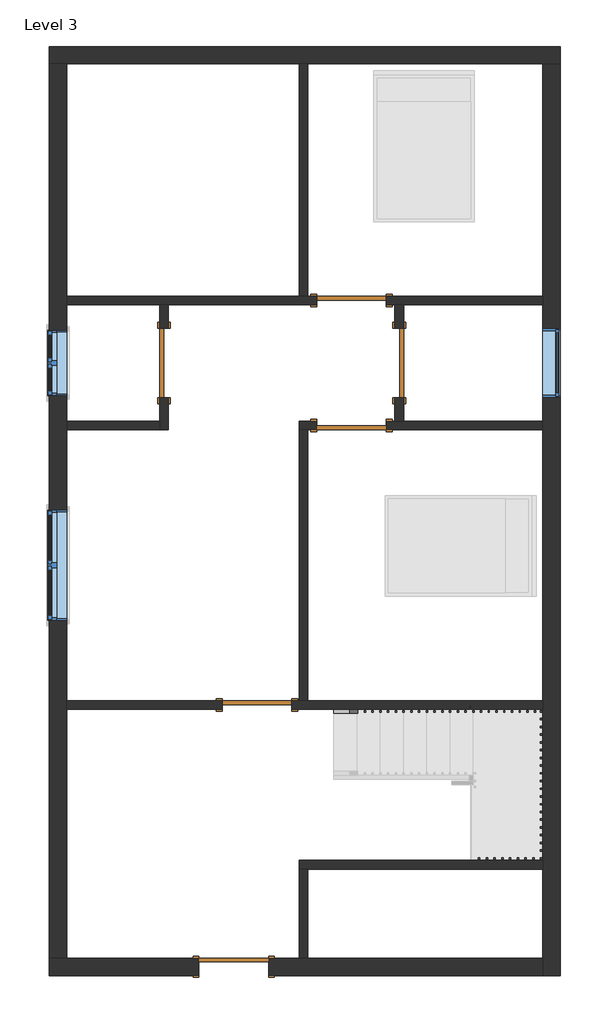
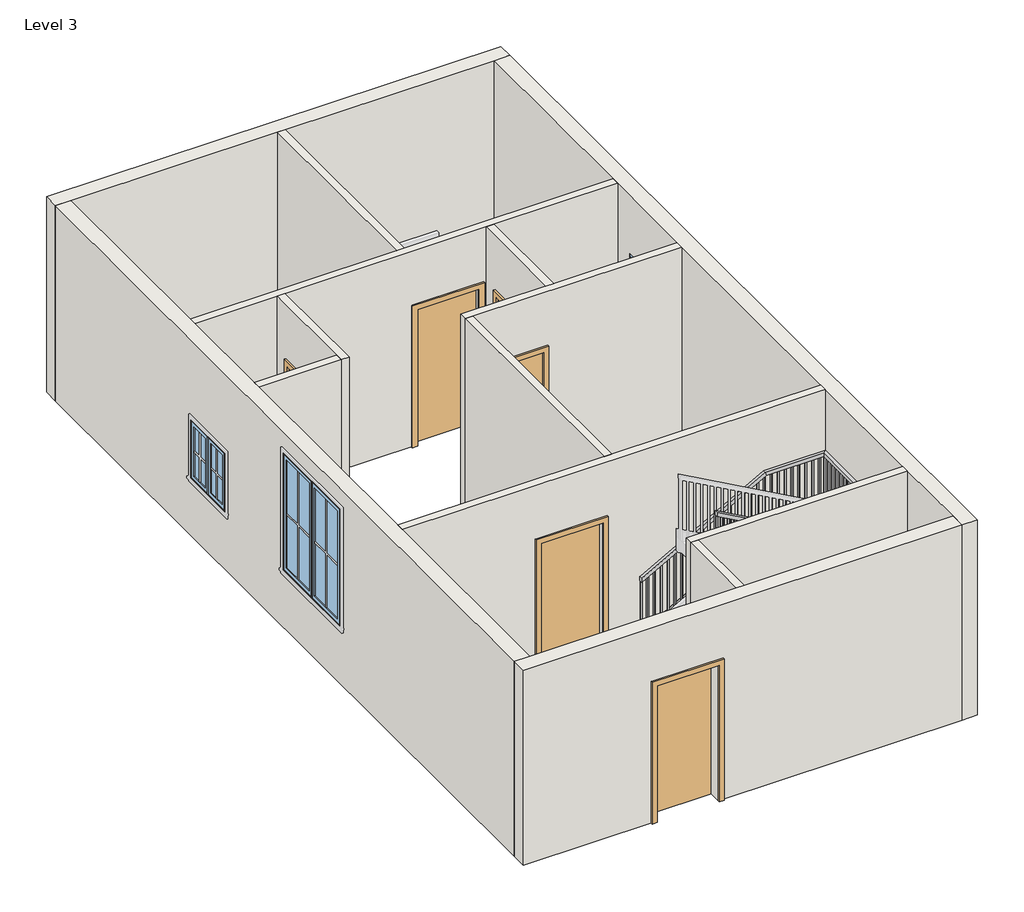
# One storey, part 1 of 2: 14 walls, 6 doors, 3 windows, 1 railing.
"""IFC4 building model written with IfcOpenShell, lengths in millimetres."""

from ifc_helpers import new_model, si_unit, frame, origin, place, context, project, spatial, polyline, outline, extrude, faceted_brep, transform, mapped, element, save
from components import door_305aa2a5, door_e5f9f3c4, door_a90ba1ad, window_c1f32544, window_339605e1, window_9ac97e1a

model = new_model("IFC4")

# Units and contexts
model_context = context("Model", 3, world=origin())
ifc_project = project(units=[si_unit("LENGTHUNIT", "METRE", prefix="MILLI")], contexts=[model_context])

# Site, building, storey
site = spatial("IfcSite", under=ifc_project)
building = spatial("IfcBuilding", under=site)
storey = spatial("IfcBuildingStorey", under=building, Name="Level 3", Elevation=3200.4)

# Doors
placement = place(None, origin())
door_shape = door_305aa2a5(model_context)
element("IfcDoor", 1, ObjectType="Single-Flush : 36\" x 84\"", at=placement, inside=storey, context=model_context, shape_type="MappedRepresentation", body=[
    mapped(door_shape, transform((-650.940747, 3300.4435985, 3200.4), x_axis=(-1.0, 0.0, 0.0), y_axis=(0.0, -1.0, 0.0), z_axis=(0.0, 0.0, 1.0))),
])
element("IfcDoor", 2, ObjectType="Single-Flush : 36\" x 84\"", at=placement, inside=storey, context=model_context, shape_type="MappedRepresentation", body=[
    mapped(door_shape, transform((-22.290747, 2481.2935985, 3200.4), x_axis=(0.0, 1.0, 0.0), y_axis=(-1.0, 0.0, 0.0), z_axis=(0.0, 0.0, 1.0))),
])
door_2_shape = door_e5f9f3c4(model_context)
element("IfcDoor", 3, ObjectType="Single-Flush : 36\" x 84\"", at=placement, inside=storey, context=model_context, shape_type="MappedRepresentation", body=[
    mapped(door_2_shape, transform((-650.940747, 1662.1435985, 3200.4), x_axis=(-1.0, 0.0, 0.0), y_axis=(0.0, -1.0, 0.0), z_axis=(0.0, 0.0, 1.0))),
])
element("IfcDoor", 4, ObjectType="Single-Flush : 36\" x 84\"", at=placement, inside=storey, context=model_context, shape_type="MappedRepresentation", body=[
    mapped(door_2_shape, transform((-3108.390747, 2481.2935985, 3200.4), x_axis=(0.0, 1.0, 0.0), y_axis=(-1.0, 0.0, 0.0), z_axis=(0.0, 0.0, 1.0))),
])
element("IfcDoor", 5, ObjectType="Single-Flush : 36\" x 84\"", at=placement, inside=storey, context=model_context, shape_type="MappedRepresentation", body=[
    mapped(door_2_shape, transform((-1889.190747, -2008.1564015, 3200.4), x_axis=(1.0, 0.0, 0.0), y_axis=(0.0, 1.0, 0.0), z_axis=(0.0, 0.0, 1.0))),
])
door_3_shape = door_a90ba1ad(model_context)
element("IfcDoor", 6, ObjectType="Single-Flush : 36\" x 84\"", at=placement, inside=storey, context=model_context, shape_type="MappedRepresentation", body=[
    mapped(door_3_shape, transform((-2193.990747, -5443.5064015, 3200.4), x_axis=(-1.0, 0.0, 0.0), y_axis=(0.0, -1.0, 0.0), z_axis=(0.0, 0.0, 1.0))),
])

# Railing
element("IfcRailing", 7, ObjectType="Handrail - Rectangular", at=placement, inside=storey, context=model_context, shape_type="SolidModel", body=[
    faceted_brep([(-879.540747, -2065.3064015, 4284.1333333), (-879.540747, -2065.3064015, 4226.020221), (-879.540747, -2116.1064015, 4226.020221), (-879.540747, -2116.1064015, 4284.1333333), (949.259253, -2065.3064015, 5300.1333333), (962.4228552, -2065.3064015, 5249.3333333), (962.4228552, -2116.1064015, 5249.3333333), (949.259253, -2116.1064015, 5300.1333333), (1863.659253, -2065.3064015, 5300.1333333), (1863.659253, -2065.3064015, 5249.3333333), (1812.859253, -2116.1064015, 5249.3333333), (1812.859253, -2116.1064015, 5300.1333333), (1863.659253, -4046.5064015, 5300.1333333), (1863.659253, -4046.5064015, 5249.3333333), (1812.859253, -3995.7064015, 5249.3333333), (1812.859253, -3995.7064015, 5300.1333333), (1254.059253, -4046.5064015, 5300.1333333), (1240.8956508, -4046.5064015, 5249.3333333), (1240.8956508, -3995.7064015, 5249.3333333), (1254.059253, -3995.7064015, 5300.1333333), (-879.540747, -4046.5064015, 6485.4666667), (-879.540747, -3995.7064015, 6485.4666667), (-879.540747, -3995.7064015, 6427.3535543), (-879.540747, -4046.5064015, 6427.3535543)], [[[0, 1, 2, 3]], [[1, 0, 4, 5]], [[2, 1, 5, 6]], [[3, 2, 6, 7]], [[0, 3, 7, 4]], [[5, 4, 8, 9]], [[6, 5, 9, 10]], [[7, 6, 10, 11]], [[4, 7, 11, 8]], [[9, 8, 12, 13]], [[10, 9, 13, 14]], [[11, 10, 14, 15]], [[8, 11, 15, 12]], [[13, 12, 16, 17]], [[14, 13, 17, 18]], [[15, 14, 18, 19]], [[12, 15, 19, 16]], [[20, 21, 22, 23]], [[17, 16, 20, 23]], [[18, 17, 23, 22]], [[19, 18, 22, 21]], [[16, 19, 21, 20]]]),
    extrude(outline(polyline([(6390.3118876, -812.865747), (5401.7333333, -812.865747), (5401.7333333, -793.815747), (6379.7285543, -793.815747), (6390.3118876, -812.865747)])), frame((0.0, -4030.6314015, 0.0), z_axis=(0.0, 1.0, 0.0), x_axis=(0.0, 0.0, 1.0)), (0.0, 0.0, 1.0), 19.05),
    extrude(outline(polyline([(6333.8674432, -711.265747), (5401.7333333, -711.265747), (5401.7333333, -692.215747), (6323.2841099, -692.215747), (6333.8674432, -711.265747)])), frame((0.0, -4030.6314015, 0.0), z_axis=(0.0, 1.0, 0.0), x_axis=(0.0, 0.0, 1.0)), (0.0, 0.0, 1.0), 19.05),
    extrude(outline(polyline([(6277.4229988, -609.665747), (5401.7333333, -609.665747), (5401.7333333, -590.615747), (6266.8396654, -590.615747), (6277.4229988, -609.665747)])), frame((0.0, -4030.6314015, 0.0), z_axis=(0.0, 1.0, 0.0), x_axis=(0.0, 0.0, 1.0)), (0.0, 0.0, 1.0), 19.05),
    extrude(outline(polyline([(6220.9785543, -508.065747), (5232.4, -508.065747), (5232.4, -489.015747), (6210.395221, -489.015747), (6220.9785543, -508.065747)])), frame((0.0, -4030.6314015, 0.0), z_axis=(0.0, 1.0, 0.0), x_axis=(0.0, 0.0, 1.0)), (0.0, 0.0, 1.0), 19.05),
    extrude(outline(polyline([(6164.5341099, -406.465747), (5232.4, -406.465747), (5232.4, -387.415747), (6153.9507765, -387.415747), (6164.5341099, -406.465747)])), frame((0.0, -4030.6314015, 0.0), z_axis=(0.0, 1.0, 0.0), x_axis=(0.0, 0.0, 1.0)), (0.0, 0.0, 1.0), 19.05),
    extrude(outline(polyline([(6108.0896654, -304.865747), (5232.4, -304.865747), (5232.4, -285.815747), (6097.5063321, -285.815747), (6108.0896654, -304.865747)])), frame((0.0, -4030.6314015, 0.0), z_axis=(0.0, 1.0, 0.0), x_axis=(0.0, 0.0, 1.0)), (0.0, 0.0, 1.0), 19.05),
    extrude(outline(polyline([(6051.645221, -203.265747), (5063.0666667, -203.265747), (5063.0666667, -184.215747), (6041.0618876, -184.215747), (6051.645221, -203.265747)])), frame((0.0, -4030.6314015, 0.0), z_axis=(0.0, 1.0, 0.0), x_axis=(0.0, 0.0, 1.0)), (0.0, 0.0, 1.0), 19.05),
    extrude(outline(polyline([(5995.2007765, -101.665747), (5063.0666667, -101.665747), (5063.0666667, -82.615747), (5984.6174432, -82.615747), (5995.2007765, -101.665747)])), frame((0.0, -4030.6314015, 0.0), z_axis=(0.0, 1.0, 0.0), x_axis=(0.0, 0.0, 1.0)), (0.0, 0.0, 1.0), 19.05),
    extrude(outline(polyline([(5938.7563321, -0.065747), (5063.0666667, -0.065747), (5063.0666667, 18.984253), (5928.1729988, 18.984253), (5938.7563321, -0.065747)])), frame((0.0, -4030.6314015, 0.0), z_axis=(0.0, 1.0, 0.0), x_axis=(0.0, 0.0, 1.0)), (0.0, 0.0, 1.0), 19.05),
    extrude(outline(polyline([(5882.3118876, 101.534253), (4893.7333333, 101.534253), (4893.7333333, 120.584253), (5871.7285543, 120.584253), (5882.3118876, 101.534253)])), frame((0.0, -4030.6314015, 0.0), z_axis=(0.0, 1.0, 0.0), x_axis=(0.0, 0.0, 1.0)), (0.0, 0.0, 1.0), 19.05),
    extrude(outline(polyline([(5825.8674432, 203.134253), (4893.7333333, 203.134253), (4893.7333333, 222.184253), (5815.2841099, 222.184253), (5825.8674432, 203.134253)])), frame((0.0, -4030.6314015, 0.0), z_axis=(0.0, 1.0, 0.0), x_axis=(0.0, 0.0, 1.0)), (0.0, 0.0, 1.0), 19.05),
    extrude(outline(polyline([(5769.4229988, 304.734253), (4893.7333333, 304.734253), (4893.7333333, 323.784253), (5758.8396654, 323.784253), (5769.4229988, 304.734253)])), frame((0.0, -4030.6314015, 0.0), z_axis=(0.0, 1.0, 0.0), x_axis=(0.0, 0.0, 1.0)), (0.0, 0.0, 1.0), 19.05),
    extrude(outline(polyline([(5712.9785543, 406.334253), (4724.4, 406.334253), (4724.4, 425.384253), (5702.395221, 425.384253), (5712.9785543, 406.334253)])), frame((0.0, -4030.6314015, 0.0), z_axis=(0.0, 1.0, 0.0), x_axis=(0.0, 0.0, 1.0)), (0.0, 0.0, 1.0), 19.05),
    extrude(outline(polyline([(5656.5341099, 507.934253), (4724.4, 507.934253), (4724.4, 526.984253), (5645.9507765, 526.984253), (5656.5341099, 507.934253)])), frame((0.0, -4030.6314015, 0.0), z_axis=(0.0, 1.0, 0.0), x_axis=(0.0, 0.0, 1.0)), (0.0, 0.0, 1.0), 19.05),
    extrude(outline(polyline([(5600.0896654, 609.534253), (4724.4, 609.534253), (4724.4, 628.584253), (5589.5063321, 628.584253), (5600.0896654, 609.534253)])), frame((0.0, -4030.6314015, 0.0), z_axis=(0.0, 1.0, 0.0), x_axis=(0.0, 0.0, 1.0)), (0.0, 0.0, 1.0), 19.05),
    extrude(outline(polyline([(5543.645221, 711.134253), (4555.0666667, 711.134253), (4555.0666667, 730.184253), (5533.0618876, 730.184253), (5543.645221, 711.134253)])), frame((0.0, -4030.6314015, 0.0), z_axis=(0.0, 1.0, 0.0), x_axis=(0.0, 0.0, 1.0)), (0.0, 0.0, 1.0), 19.05),
    extrude(outline(polyline([(5487.2007765, 812.734253), (4555.0666667, 812.734253), (4555.0666667, 831.784253), (5476.6174432, 831.784253), (5487.2007765, 812.734253)])), frame((0.0, -4030.6314015, 0.0), z_axis=(0.0, 1.0, 0.0), x_axis=(0.0, 0.0, 1.0)), (0.0, 0.0, 1.0), 19.05),
    extrude(outline(polyline([(5430.7563321, 914.334253), (4555.0666667, 914.334253), (4555.0666667, 933.384253), (5420.1729988, 933.384253), (5430.7563321, 914.334253)])), frame((0.0, -4030.6314015, 0.0), z_axis=(0.0, 1.0, 0.0), x_axis=(0.0, 0.0, 1.0)), (0.0, 0.0, 1.0), 19.05),
    extrude(outline(polyline([(5374.3118876, 1015.934253), (4385.7333333, 1015.934253), (4385.7333333, 1034.984253), (5363.7285543, 1034.984253), (5374.3118876, 1015.934253)])), frame((0.0, -4030.6314015, 0.0), z_axis=(0.0, 1.0, 0.0), x_axis=(0.0, 0.0, 1.0)), (0.0, 0.0, 1.0), 19.05),
    extrude(outline(polyline([(5317.8674432, 1117.534253), (4385.7333333, 1117.534253), (4385.7333333, 1136.584253), (5307.2841099, 1136.584253), (5317.8674432, 1117.534253)])), frame((0.0, -4030.6314015, 0.0), z_axis=(0.0, 1.0, 0.0), x_axis=(0.0, 0.0, 1.0)), (0.0, 0.0, 1.0), 19.05),
    extrude(outline(polyline([(5261.4229988, 1219.134253), (4385.7333333, 1219.134253), (4385.7333333, 1238.184253), (5250.8396654, 1238.184253), (5261.4229988, 1219.134253)])), frame((0.0, -4030.6314015, 0.0), z_axis=(0.0, 1.0, 0.0), x_axis=(0.0, 0.0, 1.0)), (0.0, 0.0, 1.0), 19.05),
    extrude(outline(polyline([(1339.784253, -4030.6314015), (1320.734253, -4030.6314015), (1320.734253, -4011.5814015), (1339.784253, -4011.5814015), (1339.784253, -4030.6314015)])), frame((0.0, 0.0, 4385.7333333), z_axis=(0.0, 0.0, 1.0), x_axis=(1.0, 0.0, 0.0)), (0.0, 0.0, 1.0), 863.6),
    extrude(outline(polyline([(1441.384253, -4030.6314015), (1422.334253, -4030.6314015), (1422.334253, -4011.5814015), (1441.384253, -4011.5814015), (1441.384253, -4030.6314015)])), frame((0.0, 0.0, 4385.7333333), z_axis=(0.0, 0.0, 1.0), x_axis=(1.0, 0.0, 0.0)), (0.0, 0.0, 1.0), 863.6),
    extrude(outline(polyline([(1542.984253, -4030.6314015), (1523.934253, -4030.6314015), (1523.934253, -4011.5814015), (1542.984253, -4011.5814015), (1542.984253, -4030.6314015)])), frame((0.0, 0.0, 4385.7333333), z_axis=(0.0, 0.0, 1.0), x_axis=(1.0, 0.0, 0.0)), (0.0, 0.0, 1.0), 863.6),
    extrude(outline(polyline([(1644.584253, -4030.6314015), (1625.534253, -4030.6314015), (1625.534253, -4011.5814015), (1644.584253, -4011.5814015), (1644.584253, -4030.6314015)])), frame((0.0, 0.0, 4385.7333333), z_axis=(0.0, 0.0, 1.0), x_axis=(1.0, 0.0, 0.0)), (0.0, 0.0, 1.0), 863.6),
    extrude(outline(polyline([(1746.184253, -4030.6314015), (1727.134253, -4030.6314015), (1727.134253, -4011.5814015), (1746.184253, -4011.5814015), (1746.184253, -4030.6314015)])), frame((0.0, 0.0, 4385.7333333), z_axis=(0.0, 0.0, 1.0), x_axis=(1.0, 0.0, 0.0)), (0.0, 0.0, 1.0), 863.6),
    extrude(outline(polyline([(1847.784253, -3909.9814015), (1847.784253, -3929.0314015), (1828.734253, -3929.0314015), (1828.734253, -3909.9814015), (1847.784253, -3909.9814015)])), frame((0.0, 0.0, 4385.7333333), z_axis=(0.0, 0.0, 1.0), x_axis=(1.0, 0.0, 0.0)), (0.0, 0.0, 1.0), 863.6),
    extrude(outline(polyline([(1847.784253, -3808.3814015), (1847.784253, -3827.4314015), (1828.734253, -3827.4314015), (1828.734253, -3808.3814015), (1847.784253, -3808.3814015)])), frame((0.0, 0.0, 4385.7333333), z_axis=(0.0, 0.0, 1.0), x_axis=(1.0, 0.0, 0.0)), (0.0, 0.0, 1.0), 863.6),
    extrude(outline(polyline([(1847.784253, -3706.7814015), (1847.784253, -3725.8314015), (1828.734253, -3725.8314015), (1828.734253, -3706.7814015), (1847.784253, -3706.7814015)])), frame((0.0, 0.0, 4385.7333333), z_axis=(0.0, 0.0, 1.0), x_axis=(1.0, 0.0, 0.0)), (0.0, 0.0, 1.0), 863.6),
    extrude(outline(polyline([(1847.784253, -3605.1814015), (1847.784253, -3624.2314015), (1828.734253, -3624.2314015), (1828.734253, -3605.1814015), (1847.784253, -3605.1814015)])), frame((0.0, 0.0, 4385.7333333), z_axis=(0.0, 0.0, 1.0), x_axis=(1.0, 0.0, 0.0)), (0.0, 0.0, 1.0), 863.6),
    extrude(outline(polyline([(1847.784253, -3503.5814015), (1847.784253, -3522.6314015), (1828.734253, -3522.6314015), (1828.734253, -3503.5814015), (1847.784253, -3503.5814015)])), frame((0.0, 0.0, 4385.7333333), z_axis=(0.0, 0.0, 1.0), x_axis=(1.0, 0.0, 0.0)), (0.0, 0.0, 1.0), 863.6),
    extrude(outline(polyline([(1847.784253, -3401.9814015), (1847.784253, -3421.0314015), (1828.734253, -3421.0314015), (1828.734253, -3401.9814015), (1847.784253, -3401.9814015)])), frame((0.0, 0.0, 4385.7333333), z_axis=(0.0, 0.0, 1.0), x_axis=(1.0, 0.0, 0.0)), (0.0, 0.0, 1.0), 863.6),
    extrude(outline(polyline([(1847.784253, -3300.3814015), (1847.784253, -3319.4314015), (1828.734253, -3319.4314015), (1828.734253, -3300.3814015), (1847.784253, -3300.3814015)])), frame((0.0, 0.0, 4385.7333333), z_axis=(0.0, 0.0, 1.0), x_axis=(1.0, 0.0, 0.0)), (0.0, 0.0, 1.0), 863.6),
    extrude(outline(polyline([(1847.784253, -3198.7814015), (1847.784253, -3217.8314015), (1828.734253, -3217.8314015), (1828.734253, -3198.7814015), (1847.784253, -3198.7814015)])), frame((0.0, 0.0, 4385.7333333), z_axis=(0.0, 0.0, 1.0), x_axis=(1.0, 0.0, 0.0)), (0.0, 0.0, 1.0), 863.6),
    extrude(outline(polyline([(1847.784253, -3097.1814015), (1847.784253, -3116.2314015), (1828.734253, -3116.2314015), (1828.734253, -3097.1814015), (1847.784253, -3097.1814015)])), frame((0.0, 0.0, 4385.7333333), z_axis=(0.0, 0.0, 1.0), x_axis=(1.0, 0.0, 0.0)), (0.0, 0.0, 1.0), 863.6),
    extrude(outline(polyline([(1847.784253, -2995.5814015), (1847.784253, -3014.6314015), (1828.734253, -3014.6314015), (1828.734253, -2995.5814015), (1847.784253, -2995.5814015)])), frame((0.0, 0.0, 4385.7333333), z_axis=(0.0, 0.0, 1.0), x_axis=(1.0, 0.0, 0.0)), (0.0, 0.0, 1.0), 863.6),
    extrude(outline(polyline([(1847.784253, -2893.9814015), (1847.784253, -2913.0314015), (1828.734253, -2913.0314015), (1828.734253, -2893.9814015), (1847.784253, -2893.9814015)])), frame((0.0, 0.0, 4385.7333333), z_axis=(0.0, 0.0, 1.0), x_axis=(1.0, 0.0, 0.0)), (0.0, 0.0, 1.0), 863.6),
    extrude(outline(polyline([(1847.784253, -2792.3814015), (1847.784253, -2811.4314015), (1828.734253, -2811.4314015), (1828.734253, -2792.3814015), (1847.784253, -2792.3814015)])), frame((0.0, 0.0, 4385.7333333), z_axis=(0.0, 0.0, 1.0), x_axis=(1.0, 0.0, 0.0)), (0.0, 0.0, 1.0), 863.6),
    extrude(outline(polyline([(1847.784253, -2690.7814015), (1847.784253, -2709.8314015), (1828.734253, -2709.8314015), (1828.734253, -2690.7814015), (1847.784253, -2690.7814015)])), frame((0.0, 0.0, 4385.7333333), z_axis=(0.0, 0.0, 1.0), x_axis=(1.0, 0.0, 0.0)), (0.0, 0.0, 1.0), 863.6),
    extrude(outline(polyline([(1847.784253, -2589.1814015), (1847.784253, -2608.2314015), (1828.734253, -2608.2314015), (1828.734253, -2589.1814015), (1847.784253, -2589.1814015)])), frame((0.0, 0.0, 4385.7333333), z_axis=(0.0, 0.0, 1.0), x_axis=(1.0, 0.0, 0.0)), (0.0, 0.0, 1.0), 863.6),
    extrude(outline(polyline([(1847.784253, -2487.5814015), (1847.784253, -2506.6314015), (1828.734253, -2506.6314015), (1828.734253, -2487.5814015), (1847.784253, -2487.5814015)])), frame((0.0, 0.0, 4385.7333333), z_axis=(0.0, 0.0, 1.0), x_axis=(1.0, 0.0, 0.0)), (0.0, 0.0, 1.0), 863.6),
    extrude(outline(polyline([(1847.784253, -2385.9814015), (1847.784253, -2405.0314015), (1828.734253, -2405.0314015), (1828.734253, -2385.9814015), (1847.784253, -2385.9814015)])), frame((0.0, 0.0, 4385.7333333), z_axis=(0.0, 0.0, 1.0), x_axis=(1.0, 0.0, 0.0)), (0.0, 0.0, 1.0), 863.6),
    extrude(outline(polyline([(1847.784253, -2284.3814015), (1847.784253, -2303.4314015), (1828.734253, -2303.4314015), (1828.734253, -2284.3814015), (1847.784253, -2284.3814015)])), frame((0.0, 0.0, 4385.7333333), z_axis=(0.0, 0.0, 1.0), x_axis=(1.0, 0.0, 0.0)), (0.0, 0.0, 1.0), 863.6),
    extrude(outline(polyline([(1847.784253, -2182.7814015), (1847.784253, -2201.8314015), (1828.734253, -2201.8314015), (1828.734253, -2182.7814015), (1847.784253, -2182.7814015)])), frame((0.0, 0.0, 4385.7333333), z_axis=(0.0, 0.0, 1.0), x_axis=(1.0, 0.0, 0.0)), (0.0, 0.0, 1.0), 863.6),
    extrude(outline(polyline([(1752.534253, -2081.1814015), (1771.584253, -2081.1814015), (1771.584253, -2100.2314015), (1752.534253, -2100.2314015), (1752.534253, -2081.1814015)])), frame((0.0, 0.0, 4385.7333333), z_axis=(0.0, 0.0, 1.0), x_axis=(1.0, 0.0, 0.0)), (0.0, 0.0, 1.0), 863.6),
    extrude(outline(polyline([(1650.934253, -2081.1814015), (1669.984253, -2081.1814015), (1669.984253, -2100.2314015), (1650.934253, -2100.2314015), (1650.934253, -2081.1814015)])), frame((0.0, 0.0, 4385.7333333), z_axis=(0.0, 0.0, 1.0), x_axis=(1.0, 0.0, 0.0)), (0.0, 0.0, 1.0), 863.6),
    extrude(outline(polyline([(1549.334253, -2081.1814015), (1568.384253, -2081.1814015), (1568.384253, -2100.2314015), (1549.334253, -2100.2314015), (1549.334253, -2081.1814015)])), frame((0.0, 0.0, 4385.7333333), z_axis=(0.0, 0.0, 1.0), x_axis=(1.0, 0.0, 0.0)), (0.0, 0.0, 1.0), 863.6),
    extrude(outline(polyline([(1447.734253, -2081.1814015), (1466.784253, -2081.1814015), (1466.784253, -2100.2314015), (1447.734253, -2100.2314015), (1447.734253, -2081.1814015)])), frame((0.0, 0.0, 4385.7333333), z_axis=(0.0, 0.0, 1.0), x_axis=(1.0, 0.0, 0.0)), (0.0, 0.0, 1.0), 863.6),
    extrude(outline(polyline([(1346.134253, -2081.1814015), (1365.184253, -2081.1814015), (1365.184253, -2100.2314015), (1346.134253, -2100.2314015), (1346.134253, -2081.1814015)])), frame((0.0, 0.0, 4385.7333333), z_axis=(0.0, 0.0, 1.0), x_axis=(1.0, 0.0, 0.0)), (0.0, 0.0, 1.0), 863.6),
    extrude(outline(polyline([(1244.534253, -2081.1814015), (1263.584253, -2081.1814015), (1263.584253, -2100.2314015), (1244.534253, -2100.2314015), (1244.534253, -2081.1814015)])), frame((0.0, 0.0, 4385.7333333), z_axis=(0.0, 0.0, 1.0), x_axis=(1.0, 0.0, 0.0)), (0.0, 0.0, 1.0), 863.6),
    extrude(outline(polyline([(1142.934253, -2081.1814015), (1161.984253, -2081.1814015), (1161.984253, -2100.2314015), (1142.934253, -2100.2314015), (1142.934253, -2081.1814015)])), frame((0.0, 0.0, 4385.7333333), z_axis=(0.0, 0.0, 1.0), x_axis=(1.0, 0.0, 0.0)), (0.0, 0.0, 1.0), 863.6),
    extrude(outline(polyline([(1041.334253, -2081.1814015), (1060.384253, -2081.1814015), (1060.384253, -2100.2314015), (1041.334253, -2100.2314015), (1041.334253, -2081.1814015)])), frame((0.0, 0.0, 4385.7333333), z_axis=(0.0, 0.0, 1.0), x_axis=(1.0, 0.0, 0.0)), (0.0, 0.0, 1.0), 863.6),
    extrude(outline(polyline([(5236.7285543, 939.734253), (4385.7333333, 939.734253), (4385.7333333, 958.784253), (5247.3118876, 958.784253), (5236.7285543, 939.734253)])), frame((0.0, -2100.2314015, 0.0), z_axis=(0.0, 1.0, 0.0), x_axis=(0.0, 0.0, 1.0)), (0.0, 0.0, 1.0), 19.05),
    extrude(outline(polyline([(5180.2841099, 838.134253), (4216.4, 838.134253), (4216.4, 857.184253), (5190.8674432, 857.184253), (5180.2841099, 838.134253)])), frame((0.0, -2100.2314015, 0.0), z_axis=(0.0, 1.0, 0.0), x_axis=(0.0, 0.0, 1.0)), (0.0, 0.0, 1.0), 19.05),
    extrude(outline(polyline([(5123.8396654, 736.534253), (4216.4, 736.534253), (4216.4, 755.584253), (5134.4229988, 755.584253), (5123.8396654, 736.534253)])), frame((0.0, -2100.2314015, 0.0), z_axis=(0.0, 1.0, 0.0), x_axis=(0.0, 0.0, 1.0)), (0.0, 0.0, 1.0), 19.05),
    extrude(outline(polyline([(5067.395221, 634.934253), (4216.4, 634.934253), (4216.4, 653.984253), (5077.9785543, 653.984253), (5067.395221, 634.934253)])), frame((0.0, -2100.2314015, 0.0), z_axis=(0.0, 1.0, 0.0), x_axis=(0.0, 0.0, 1.0)), (0.0, 0.0, 1.0), 19.05),
    extrude(outline(polyline([(5010.9507765, 533.334253), (4047.0666667, 533.334253), (4047.0666667, 552.384253), (5021.5341099, 552.384253), (5010.9507765, 533.334253)])), frame((0.0, -2100.2314015, 0.0), z_axis=(0.0, 1.0, 0.0), x_axis=(0.0, 0.0, 1.0)), (0.0, 0.0, 1.0), 19.05),
    extrude(outline(polyline([(4954.5063321, 431.734253), (4047.0666667, 431.734253), (4047.0666667, 450.784253), (4965.0896654, 450.784253), (4954.5063321, 431.734253)])), frame((0.0, -2100.2314015, 0.0), z_axis=(0.0, 1.0, 0.0), x_axis=(0.0, 0.0, 1.0)), (0.0, 0.0, 1.0), 19.05),
    extrude(outline(polyline([(4898.0618876, 330.134253), (4047.0666667, 330.134253), (4047.0666667, 349.184253), (4908.645221, 349.184253), (4898.0618876, 330.134253)])), frame((0.0, -2100.2314015, 0.0), z_axis=(0.0, 1.0, 0.0), x_axis=(0.0, 0.0, 1.0)), (0.0, 0.0, 1.0), 19.05),
    extrude(outline(polyline([(4841.6174432, 228.534253), (3877.7333333, 228.534253), (3877.7333333, 247.584253), (4852.2007765, 247.584253), (4841.6174432, 228.534253)])), frame((0.0, -2100.2314015, 0.0), z_axis=(0.0, 1.0, 0.0), x_axis=(0.0, 0.0, 1.0)), (0.0, 0.0, 1.0), 19.05),
    extrude(outline(polyline([(4785.1729988, 126.934253), (3877.7333333, 126.934253), (3877.7333333, 145.984253), (4795.7563321, 145.984253), (4785.1729988, 126.934253)])), frame((0.0, -2100.2314015, 0.0), z_axis=(0.0, 1.0, 0.0), x_axis=(0.0, 0.0, 1.0)), (0.0, 0.0, 1.0), 19.05),
    extrude(outline(polyline([(4728.7285543, 25.334253), (3877.7333333, 25.334253), (3877.7333333, 44.384253), (4739.3118876, 44.384253), (4728.7285543, 25.334253)])), frame((0.0, -2100.2314015, 0.0), z_axis=(0.0, 1.0, 0.0), x_axis=(0.0, 0.0, 1.0)), (0.0, 0.0, 1.0), 19.05),
    extrude(outline(polyline([(4672.2841099, -76.265747), (3708.4, -76.265747), (3708.4, -57.215747), (4682.8674432, -57.215747), (4672.2841099, -76.265747)])), frame((0.0, -2100.2314015, 0.0), z_axis=(0.0, 1.0, 0.0), x_axis=(0.0, 0.0, 1.0)), (0.0, 0.0, 1.0), 19.05),
    extrude(outline(polyline([(4615.8396654, -177.865747), (3708.4, -177.865747), (3708.4, -158.815747), (4626.4229988, -158.815747), (4615.8396654, -177.865747)])), frame((0.0, -2100.2314015, 0.0), z_axis=(0.0, 1.0, 0.0), x_axis=(0.0, 0.0, 1.0)), (0.0, 0.0, 1.0), 19.05),
    extrude(outline(polyline([(4559.395221, -279.465747), (3708.4, -279.465747), (3708.4, -260.415747), (4569.9785543, -260.415747), (4559.395221, -279.465747)])), frame((0.0, -2100.2314015, 0.0), z_axis=(0.0, 1.0, 0.0), x_axis=(0.0, 0.0, 1.0)), (0.0, 0.0, 1.0), 19.05),
    extrude(outline(polyline([(4502.9507765, -381.065747), (3539.0666667, -381.065747), (3539.0666667, -362.015747), (4513.5341099, -362.015747), (4502.9507765, -381.065747)])), frame((0.0, -2100.2314015, 0.0), z_axis=(0.0, 1.0, 0.0), x_axis=(0.0, 0.0, 1.0)), (0.0, 0.0, 1.0), 19.05),
    extrude(outline(polyline([(4446.5063321, -482.665747), (3539.0666667, -482.665747), (3539.0666667, -463.615747), (4457.0896654, -463.615747), (4446.5063321, -482.665747)])), frame((0.0, -2100.2314015, 0.0), z_axis=(0.0, 1.0, 0.0), x_axis=(0.0, 0.0, 1.0)), (0.0, 0.0, 1.0), 19.05),
    extrude(outline(polyline([(4390.0618876, -584.265747), (3539.0666667, -584.265747), (3539.0666667, -565.215747), (4400.645221, -565.215747), (4390.0618876, -584.265747)])), frame((0.0, -2100.2314015, 0.0), z_axis=(0.0, 1.0, 0.0), x_axis=(0.0, 0.0, 1.0)), (0.0, 0.0, 1.0), 19.05),
    extrude(outline(polyline([(4333.6174432, -685.865747), (3369.7333333, -685.865747), (3369.7333333, -666.815747), (4344.2007765, -666.815747), (4333.6174432, -685.865747)])), frame((0.0, -2100.2314015, 0.0), z_axis=(0.0, 1.0, 0.0), x_axis=(0.0, 0.0, 1.0)), (0.0, 0.0, 1.0), 19.05),
    extrude(outline(polyline([(4277.1729988, -787.465747), (3369.7333333, -787.465747), (3369.7333333, -768.415747), (4287.7563321, -768.415747), (4277.1729988, -787.465747)])), frame((0.0, -2100.2314015, 0.0), z_axis=(0.0, 1.0, 0.0), x_axis=(0.0, 0.0, 1.0)), (0.0, 0.0, 1.0), 19.05),
    extrude(outline(polyline([(1847.784253, -4011.5814015), (1847.784253, -4030.6314015), (1828.734253, -4030.6314015), (1828.734253, -4011.5814015), (1847.784253, -4011.5814015)])), frame((0.0, 0.0, 4385.7333333), z_axis=(0.0, 0.0, 1.0), x_axis=(1.0, 0.0, 0.0)), (0.0, 0.0, 1.0), 863.6),
    extrude(outline(polyline([(1828.734253, -2081.1814015), (1847.784253, -2081.1814015), (1847.784253, -2100.2314015), (1828.734253, -2100.2314015), (1828.734253, -2081.1814015)])), frame((0.0, 0.0, 4385.7333333), z_axis=(0.0, 0.0, 1.0), x_axis=(1.0, 0.0, 0.0)), (0.0, 0.0, 1.0), 863.6),
    extrude(outline(polyline([(6427.3535543, -879.540747), (5401.7333333, -879.540747), (5401.7333333, -860.490747), (6416.770221, -860.490747), (6427.3535543, -879.540747)])), frame((0.0, -4030.6314015, 0.0), z_axis=(0.0, 1.0, 0.0), x_axis=(0.0, 0.0, 1.0)), (0.0, 0.0, 1.0), 19.05),
    extrude(outline(polyline([(4226.020221, -879.540747), (3369.7333333, -879.540747), (3369.7333333, -860.490747), (4236.6035543, -860.490747), (4226.020221, -879.540747)])), frame((0.0, -2100.2314015, 0.0), z_axis=(0.0, 1.0, 0.0), x_axis=(0.0, 0.0, 1.0)), (0.0, 0.0, 1.0), 19.05),
])

# Walls
element("IfcWall", 8, ObjectType="WALL4.5\"", at=placement, inside=storey, context=model_context, shape_type="SweptSolid", body=[
    extrude(outline(polyline([(-1336.740747, 3357.5935985), (-1336.740747, 6405.5935985), (-1222.440747, 6405.5935985), (-1222.440747, 3357.5935985), (-1336.740747, 3357.5935985)])), frame((0.0, 0.0, 3200.4), z_axis=(0.0, 0.0, 1.0), x_axis=(1.0, 0.0, 0.0)), (0.0, 0.0, 1.0), 3048.0),
])
element("IfcWall", 9, ObjectType="WALL4.5\"", at=placement, inside=storey, context=model_context, shape_type="Brep", body=[
    faceted_brep([(-4384.740747, 3243.2935985, 3200.4), (-3165.540747, 3243.2935985, 3200.4), (-3051.240747, 3243.2935985, 3200.4), (-1108.140747, 3243.2935985, 3200.4), (-1108.140747, 3243.2935985, 5334.0), (-193.740747, 3243.2935985, 5334.0), (-193.740747, 3243.2935985, 3200.4), (-79.440747, 3243.2935985, 3200.4), (34.859253, 3243.2935985, 3200.4), (1863.659253, 3243.2935985, 3200.4), (1863.659253, 3243.2935985, 6248.4), (34.859253, 3243.2935985, 6248.4), (-79.440747, 3243.2935985, 6248.4), (-3051.240747, 3243.2935985, 6248.4), (-3165.540747, 3243.2935985, 6248.4), (-4384.740747, 3243.2935985, 6248.4), (-1108.140747, 3357.5935985, 5334.0), (-1108.140747, 3357.5935985, 3200.4), (-1222.440747, 3357.5935985, 3200.4), (-1336.740747, 3357.5935985, 3200.4), (-4384.740747, 3357.5935985, 3200.4), (-4384.740747, 3357.5935985, 6248.4), (-1336.740747, 3357.5935985, 6248.4), (-1222.440747, 3357.5935985, 6248.4), (1863.659253, 3357.5935985, 6248.4), (1863.659253, 3357.5935985, 3200.4), (-193.740747, 3357.5935985, 3200.4), (-193.740747, 3357.5935985, 5334.0)], [[[0, 1, 2, 3, 4, 5, 6, 7, 8, 9, 10, 11, 12, 13, 14, 15]], [[16, 17, 18, 19, 20, 21, 22, 23, 24, 25, 26, 27]], [[26, 25, 9, 8, 7, 6]], [[20, 19, 18, 17, 3, 2, 1, 0]], [[10, 9, 25, 24]], [[0, 15, 21, 20]], [[4, 3, 17, 16]], [[5, 4, 16, 27]], [[6, 5, 27, 26]], [[15, 14, 13, 12, 11, 10, 24, 23, 22, 21]]]),
])
element("IfcWall", 10, ObjectType="WALL4.5\"", at=placement, inside=storey, context=model_context, shape_type="SweptSolid", body=[
    extrude(outline(polyline([(3243.2935985, 3200.4), (2938.4935985, 3200.4), (2938.4935985, 5334.0), (2024.0935985, 5334.0), (2024.0935985, 3200.4), (1719.2935985, 3200.4), (1719.2935985, 6248.4), (3243.2935985, 6248.4), (3243.2935985, 3200.4)])), frame((-79.440747, 0.0, 0.0), z_axis=(1.0, 0.0, 0.0), x_axis=(0.0, 1.0, 0.0)), (0.0, 0.0, 1.0), 114.3),
])
element("IfcWall", 11, ObjectType="WALL4.5\"", at=placement, inside=storey, context=model_context, shape_type="Brep", body=[
    faceted_brep([(-1108.140747, 1719.2935985, 5334.0), (-1108.140747, 1719.2935985, 3200.4), (-1336.740747, 1719.2935985, 3200.4), (-1336.740747, 1719.2935985, 6248.4), (-79.440747, 1719.2935985, 6248.4), (34.859253, 1719.2935985, 6248.4), (1863.659253, 1719.2935985, 6248.4), (1863.659253, 1719.2935985, 3200.4), (34.859253, 1719.2935985, 3200.4), (-79.440747, 1719.2935985, 3200.4), (-193.740747, 1719.2935985, 3200.4), (-193.740747, 1719.2935985, 5334.0), (-1336.740747, 1604.9935985, 3200.4), (-1222.440747, 1604.9935985, 3200.4), (-1108.140747, 1604.9935985, 3200.4), (-1108.140747, 1604.9935985, 5334.0), (-193.740747, 1604.9935985, 5334.0), (-193.740747, 1604.9935985, 3200.4), (1863.659253, 1604.9935985, 3200.4), (1863.659253, 1604.9935985, 6248.4), (-1222.440747, 1604.9935985, 6248.4), (-1336.740747, 1604.9935985, 6248.4)], [[[0, 1, 2, 3, 4, 5, 6, 7, 8, 9, 10, 11]], [[12, 13, 14, 15, 16, 17, 18, 19, 20, 21]], [[2, 1, 14, 13, 12]], [[10, 9, 8, 7, 18, 17]], [[7, 6, 19, 18]], [[3, 2, 12, 21]], [[15, 14, 1, 0]], [[16, 15, 0, 11]], [[17, 16, 11, 10]], [[6, 5, 4, 3, 21, 20, 19]]]),
])
element("IfcWall", 12, ObjectType="WALL4.5\"", at=placement, inside=storey, context=model_context, shape_type="SweptSolid", body=[
    extrude(outline(polyline([(-1336.740747, -1951.0064015), (-1336.740747, 1604.9935985), (-1222.440747, 1604.9935985), (-1222.440747, -1951.0064015), (-1336.740747, -1951.0064015)])), frame((0.0, 0.0, 3200.4), z_axis=(0.0, 0.0, 1.0), x_axis=(1.0, 0.0, 0.0)), (0.0, 0.0, 1.0), 3048.0),
])
element("IfcWall", 13, ObjectType="WALL4.5\"", at=placement, inside=storey, context=model_context, shape_type="Brep", body=[
    faceted_brep([(-3165.540747, 3243.2935985, 3200.4), (-3165.540747, 2938.4935985, 3200.4), (-3165.540747, 2938.4935985, 5334.0), (-3165.540747, 2024.0935985, 5334.0), (-3165.540747, 2024.0935985, 3200.4), (-3165.540747, 1719.2935985, 3200.4), (-3165.540747, 1604.9935985, 3200.4), (-3165.540747, 1604.9935985, 6248.4), (-3165.540747, 1719.2935985, 6248.4), (-3165.540747, 3243.2935985, 6248.4), (-3051.240747, 2938.4935985, 5334.0), (-3051.240747, 2938.4935985, 3200.4), (-3051.240747, 3243.2935985, 3200.4), (-3051.240747, 3243.2935985, 6248.4), (-3051.240747, 1604.9935985, 6248.4), (-3051.240747, 1604.9935985, 3200.4), (-3051.240747, 2024.0935985, 3200.4), (-3051.240747, 2024.0935985, 5334.0)], [[[0, 1, 2, 3, 4, 5, 6, 7, 8, 9]], [[10, 11, 12, 13, 14, 15, 16, 17]], [[16, 15, 6, 5, 4]], [[12, 11, 1, 0]], [[0, 9, 13, 12]], [[7, 6, 15, 14]], [[2, 1, 11, 10]], [[3, 2, 10, 17]], [[4, 3, 17, 16]], [[9, 8, 7, 14, 13]]]),
])
element("IfcWall", 14, ObjectType="WALL4.5\"", at=placement, inside=storey, context=model_context, shape_type="SweptSolid", body=[
    extrude(outline(polyline([(-4384.740747, 1719.2935985), (-3165.540747, 1719.2935985), (-3165.540747, 1604.9935985), (-4384.740747, 1604.9935985), (-4384.740747, 1719.2935985)])), frame((0.0, 0.0, 3200.4), z_axis=(0.0, 0.0, 1.0), x_axis=(1.0, 0.0, 0.0)), (0.0, 0.0, 1.0), 3048.0),
])
element("IfcWall", 15, ObjectType="WALL4.5\"", at=placement, inside=storey, context=model_context, shape_type="Brep", body=[
    faceted_brep([(-1431.990747, -2065.3064015, 5334.0), (-1431.990747, -2065.3064015, 3200.4), (1863.659253, -2065.3064015, 3200.4), (1863.659253, -2065.3064015, 6248.4), (1812.859253, -2065.3064015, 6248.4), (-879.540747, -2065.3064015, 6248.4), (-4384.740747, -2065.3064015, 6248.4), (-4384.740747, -2065.3064015, 3200.4), (-2346.390747, -2065.3064015, 3200.4), (-2346.390747, -2065.3064015, 5334.0), (1863.659253, -1951.0064015, 3200.4), (-1222.440747, -1951.0064015, 3200.4), (-1336.740747, -1951.0064015, 3200.4), (-1431.990747, -1951.0064015, 3200.4), (-1431.990747, -1951.0064015, 5334.0), (-2346.390747, -1951.0064015, 5334.0), (-2346.390747, -1951.0064015, 3200.4), (-4384.740747, -1951.0064015, 3200.4), (-4384.740747, -1951.0064015, 6248.4), (-1336.740747, -1951.0064015, 6248.4), (-1222.440747, -1951.0064015, 6248.4), (1863.659253, -1951.0064015, 6248.4)], [[[0, 1, 2, 3, 4, 5, 6, 7, 8, 9]], [[10, 11, 12, 13, 14, 15, 16, 17, 18, 19, 20, 21]], [[8, 7, 17, 16]], [[2, 1, 13, 12, 11, 10]], [[3, 2, 10, 21]], [[7, 6, 18, 17]], [[14, 13, 1, 0]], [[15, 14, 0, 9]], [[16, 15, 9, 8]], [[6, 5, 4, 3, 21, 20, 19, 18]]]),
])
element("IfcWall", 16, ObjectType="WALL4.5\"", at=placement, inside=storey, context=model_context, shape_type="Brep", body=[
    faceted_brep([(1863.659253, -4046.5064015, 3200.4), (-1336.740747, -4046.5064015, 3200.4), (-1336.740747, -4046.5064015, 6248.4), (1863.659253, -4046.5064015, 6248.4), (1863.659253, -4160.8064015, 3200.4), (1863.659253, -4160.8064015, 6248.4), (-1222.440747, -4160.8064015, 6248.4), (-1336.740747, -4160.8064015, 6248.4), (-1336.740747, -4160.8064015, 3200.4), (-1222.440747, -4160.8064015, 3200.4)], [[[0, 1, 2, 3]], [[4, 5, 6, 7, 8, 9]], [[1, 0, 4, 9, 8]], [[0, 3, 5, 4]], [[2, 1, 8, 7]], [[3, 2, 7, 6, 5]]]),
])
element("IfcWall", 17, ObjectType="WALL4.5\"", at=placement, inside=storey, context=model_context, shape_type="SweptSolid", body=[
    extrude(outline(polyline([(-1336.740747, -5329.2064015), (-1336.740747, -4160.8064015), (-1222.440747, -4160.8064015), (-1222.440747, -5329.2064015), (-1336.740747, -5329.2064015)])), frame((0.0, 0.0, 3200.4), z_axis=(0.0, 0.0, 1.0), x_axis=(1.0, 0.0, 0.0)), (0.0, 0.0, 1.0), 3048.0),
])
element("IfcWall", 18, ObjectType="WALL9\"", at=placement, inside=storey, context=model_context, shape_type="Brep", body=[
    faceted_brep([(-4613.340747, 6405.5935985, 3200.4), (-4384.740747, 6405.5935985, 3200.4), (-1336.740747, 6405.5935985, 3200.4), (-1222.440747, 6405.5935985, 3200.4), (1863.659253, 6405.5935985, 3200.4), (2092.259253, 6405.5935985, 3200.4), (2092.259253, 6405.5935985, 6248.4), (1863.659253, 6405.5935985, 6248.4), (-1222.440747, 6405.5935985, 6248.4), (-1336.740747, 6405.5935985, 6248.4), (-4384.740747, 6405.5935985, 6248.4), (-4613.340747, 6405.5935985, 6248.4), (-4613.340747, 6634.1935985, 3200.4), (-4613.340747, 6634.1935985, 6248.4), (2092.259253, 6634.1935985, 6248.4), (2092.259253, 6634.1935985, 3200.4)], [[[0, 1, 2, 3, 4, 5, 6, 7, 8, 9, 10, 11]], [[12, 13, 14, 15]], [[5, 4, 3, 2, 1, 0, 12, 15]], [[6, 5, 15, 14]], [[0, 11, 13, 12]], [[11, 10, 9, 8, 7, 6, 14, 13]]]),
])
element("IfcWall", 19, ObjectType="WALL9\"", at=placement, inside=storey, context=model_context, shape_type="Brep", body=[
    faceted_brep([(1863.659253, 6405.5935985, 3200.4), (1863.659253, 3357.5935985, 3200.4), (1863.659253, 3243.2935985, 3200.4), (1863.659253, 1719.2935985, 3200.4), (1863.659253, 1604.9935985, 3200.4), (1863.659253, -1951.0064015, 3200.4), (1863.659253, -2065.3064015, 3200.4), (1863.659253, -4046.5064015, 3200.4), (1863.659253, -4160.8064015, 3200.4), (1863.659253, -5329.2064015, 3200.4), (1863.659253, -5557.8064015, 3200.4), (1863.659253, -5557.8064015, 6248.4), (1863.659253, -5329.2064015, 6248.4), (1863.659253, -4160.8064015, 6248.4), (1863.659253, -4046.5064015, 6248.4), (1863.659253, -2065.3064015, 6248.4), (1863.659253, -1951.0064015, 6248.4), (1863.659253, 1604.9935985, 6248.4), (1863.659253, 1719.2935985, 6248.4), (1863.659253, 3243.2935985, 6248.4), (1863.659253, 3357.5935985, 6248.4), (1863.659253, 6405.5935985, 6248.4), (1863.659253, 2024.0935985, 5334.0), (1863.659253, 2024.0935985, 4114.8), (1863.659253, 2938.4935985, 4114.8), (1863.659253, 2938.4935985, 5334.0), (2092.259253, 6405.5935985, 3200.4), (2092.259253, 6405.5935985, 6248.4), (2092.259253, -5557.8064015, 6248.4), (2092.259253, -5557.8064015, 3200.4), (2092.259253, 2024.0935985, 5334.0), (2092.259253, 2938.4935985, 5334.0), (2092.259253, 2938.4935985, 4114.8), (2092.259253, 2024.0935985, 4114.8)], [[[0, 1, 2, 3, 4, 5, 6, 7, 8, 9, 10, 11, 12, 13, 14, 15, 16, 17, 18, 19, 20, 21], [22, 23, 24, 25]], [[26, 27, 28, 29], [30, 31, 32, 33]], [[10, 9, 8, 7, 6, 5, 4, 3, 2, 1, 0, 26, 29]], [[0, 21, 27, 26]], [[11, 10, 29, 28]], [[23, 22, 30, 33]], [[24, 23, 33, 32]], [[25, 24, 32, 31]], [[22, 25, 31, 30]], [[21, 20, 19, 18, 17, 16, 15, 14, 13, 12, 11, 28, 27]]]),
])
element("IfcWall", 20, ObjectType="WALL9\"", at=placement, inside=storey, context=model_context, shape_type="Brep", body=[
    faceted_brep([(-2651.190747, -5329.2064015, 5334.0), (-2651.190747, -5329.2064015, 3200.4), (-4384.740747, -5329.2064015, 3200.4), (-4613.340747, -5329.2064015, 3200.4), (-4613.340747, -5329.2064015, 6248.4), (-4384.740747, -5329.2064015, 6248.4), (-1336.740747, -5329.2064015, 6248.4), (-1222.440747, -5329.2064015, 6248.4), (1863.659253, -5329.2064015, 6248.4), (1863.659253, -5329.2064015, 3200.4), (-1222.440747, -5329.2064015, 3200.4), (-1336.740747, -5329.2064015, 3200.4), (-1736.790747, -5329.2064015, 3200.4), (-1736.790747, -5329.2064015, 5334.0), (-4613.340747, -5557.8064015, 3200.4), (-2651.190747, -5557.8064015, 3200.4), (-2651.190747, -5557.8064015, 5334.0), (-1736.790747, -5557.8064015, 5334.0), (-1736.790747, -5557.8064015, 3200.4), (1863.659253, -5557.8064015, 3200.4), (1863.659253, -5557.8064015, 6248.4), (-4613.340747, -5557.8064015, 6248.4)], [[[0, 1, 2, 3, 4, 5, 6, 7, 8, 9, 10, 11, 12, 13]], [[14, 15, 16, 17, 18, 19, 20, 21]], [[3, 2, 1, 15, 14]], [[12, 11, 10, 9, 19, 18]], [[9, 8, 20, 19]], [[4, 3, 14, 21]], [[16, 15, 1, 0]], [[17, 16, 0, 13]], [[18, 17, 13, 12]], [[8, 7, 6, 5, 4, 21, 20]]]),
])
element("IfcWall", 21, ObjectType="WALL9\"", at=placement, inside=storey, context=model_context, shape_type="Brep", body=[
    faceted_brep([(-4384.740747, -5329.2064015, 3200.4), (-4384.740747, -2065.3064015, 3200.4), (-4384.740747, -1951.0064015, 3200.4), (-4384.740747, 1604.9935985, 3200.4), (-4384.740747, 1719.2935985, 3200.4), (-4384.740747, 3243.2935985, 3200.4), (-4384.740747, 3357.5935985, 3200.4), (-4384.740747, 6405.5935985, 3200.4), (-4384.740747, 6405.5935985, 6248.4), (-4384.740747, 3357.5935985, 6248.4), (-4384.740747, 3243.2935985, 6248.4), (-4384.740747, 1719.2935985, 6248.4), (-4384.740747, 1604.9935985, 6248.4), (-4384.740747, -1951.0064015, 6248.4), (-4384.740747, -2065.3064015, 6248.4), (-4384.740747, -5329.2064015, 6248.4), (-4384.740747, 550.8935985, 5943.6), (-4384.740747, 550.8935985, 4114.8), (-4384.740747, -896.9064015, 4114.8), (-4384.740747, -896.9064015, 5943.6), (-4384.740747, 2913.0935985, 5029.2), (-4384.740747, 2913.0935985, 4114.8), (-4384.740747, 2049.4935985, 4114.8), (-4384.740747, 2049.4935985, 5029.2), (-4613.340747, -5329.2064015, 3200.4), (-4613.340747, -5329.2064015, 6248.4), (-4613.340747, 6405.5935985, 6248.4), (-4613.340747, 6405.5935985, 3200.4), (-4613.340747, 550.8935985, 5943.6), (-4613.340747, -896.9064015, 5943.6), (-4613.340747, -896.9064015, 4114.8), (-4613.340747, 550.8935985, 4114.8), (-4613.340747, 2913.0935985, 5029.2), (-4613.340747, 2049.4935985, 5029.2), (-4613.340747, 2049.4935985, 4114.8), (-4613.340747, 2913.0935985, 4114.8)], [[[0, 1, 2, 3, 4, 5, 6, 7, 8, 9, 10, 11, 12, 13, 14, 15], [16, 17, 18, 19], [20, 21, 22, 23]], [[24, 25, 26, 27], [28, 29, 30, 31], [32, 33, 34, 35]], [[7, 6, 5, 4, 3, 2, 1, 0, 24, 27]], [[8, 7, 27, 26]], [[0, 15, 25, 24]], [[17, 16, 28, 31]], [[18, 17, 31, 30]], [[19, 18, 30, 29]], [[16, 19, 29, 28]], [[21, 20, 32, 35]], [[22, 21, 35, 34]], [[23, 22, 34, 33]], [[20, 23, 33, 32]], [[15, 14, 13, 12, 11, 10, 9, 8, 26, 25]]]),
])

# Windows
window_shape = window_c1f32544(model_context)
element("IfcWindow", 22, ObjectType="Fixed : 36\" x 48\"", at=placement, inside=storey, context=model_context, shape_type="MappedRepresentation", body=[
    mapped(window_shape, transform((1977.959253, 2443.1935985, 3200.4), x_axis=(0.0, -1.0, 0.0), y_axis=(1.0, 0.0, 0.0), z_axis=(0.0, 0.0, 1.0))),
])
window_2_shape = window_339605e1(model_context)
element("IfcWindow", 23, ObjectType="Window-Casement-Double : 34\" x 36\"", at=placement, inside=storey, context=model_context, shape_type="MappedRepresentation", body=[
    mapped(window_2_shape, transform((-4499.040747, 2481.2935985, 3200.4), x_axis=(0.0, 1.0, 0.0), y_axis=(-1.0, 0.0, 0.0), z_axis=(0.0, 0.0, 1.0))),
])
window_3_shape = window_9ac97e1a(model_context)
element("IfcWindow", 24, ObjectType="Window-Casement-Double : 57\" x 72\"", at=placement, inside=storey, context=model_context, shape_type="MappedRepresentation", body=[
    mapped(window_3_shape, transform((-4499.040747, -173.0064015, 3200.4), x_axis=(0.0, 1.0, 0.0), y_axis=(-1.0, 0.0, 0.0), z_axis=(0.0, 0.0, 1.0))),
])

save(model, "model.ifc")

# Revit data of these elements
# Type "Single-Flush : 36\" x 84\""
#   Type Mark = "1"
#   Construction Type Id = "MDOOR"
#   Assembly Code = "C1020"
#   Analytic Construction = "Metal"
#   Thickness = 0' - 2"
#   Heat Transfer Coefficient (U) = 0.651978 BTU/(h·ft²·°F)
#   Height = 7' - 0"
#   Trim Projection Ext = 0' - 1"
#   Trim Projection Int = 0' - 1"
#   Trim Width = 0' - 3"
#   Width = 3' - 0"
#   Define Thermal Properties by = 1
#   Define Thermal Properties by = 1
#   Door Material = Door - Panel
#   Frame Material = Door - Frame
#   Visual Light Transmittance = 0
#   Solar Heat Gain Coefficient = 0
#   Function = (empty or 0)
#   Wall Closure = (empty or 0)
# Type "Handrail - Rectangular"
#   Assembly Code = "C2010400"
#   built-in parameter 1008612 = 0.0416667 (stored number, unit not read)
#   built-in parameter 1008611 = 0.0416667 (stored number, unit not read)
#   built-in parameter 1008609 = 0.333333 (stored number, unit not read)
#   built-in parameter 1008604 = 0.166667 (stored number, unit not read)
#   built-in parameter 1008603 = 0.166667 (stored number, unit not read)
#   Railing Height = 3' - 0"
#   built-in parameter 1008630 = 2
#   built-in parameter 1008610 = 2
#   built-in parameter 1008618 = Baluster - Square : 3/4"
# Type "WALL4.5\""
#   Assembly Code = "B2010"
#   Layers, outside or top first: 0' - 4 1/2" no material (function 1)
# Type "WALL9\""
#   Assembly Code = "B2010"
#   Layers, outside or top first: 0' - 9" no material (function 1)
# Type "Fixed : 36\" x 48\""
#   Type Mark = "1"
#   Construction Type Id = "GSP4R"
#   Assembly Code = "B2020100"
#   Analytic Construction = "1/8 in Pilkington single glazing"
#   Visual Light Transmittance = 0.9
#   Solar Heat Gain Coefficient = 0.78
#   Heat Transfer Coefficient (U) = 0.6496 BTU/(h·ft²·°F)
#   Height = 4' - 0"
#   Default Sill Height = 3' - 0"
#   Width = 3' - 0"
#   Window Inset = 0' - 0 3/4"
#   Define Thermal Properties by = 1
#   Define Thermal Properties by = 1
#   Glass Pane Material = Glass
#   Sash Material = Sash
#   Wall Closure = (empty or 0)
# Type "Window-Casement-Double : 34\" x 36\""
#   Type Mark = "14"
#   Fire Rating = "0.5h"
#   Assembly Code = "B2020100"
#   Analytic Construction = "Double glazing - domestic"
#   Frame Extension [instance default] = 0' - 0 1/4"
#   Window Inset [instance default] = 0' - 0"
#   Wall Thickness [instance default] = 0' - 6"
#   Interior Wall Closure [instance default] = 0' - 2 1/4"
#   Half Width = 1' - 5"
#   Visual Light Transmittance = 0.81
#   Thermal Resistance (R) = 1.8146 (h·ft²·°F)/BTU
#   Solar Heat Gain Coefficient = 0.76
#   Rough Width = 2' - 10 1/2"
#   Rough Height = 3' - 0 1/2"
#   Height = 3' - 0"
#   Heat Transfer Coefficient (U) = 0.5511 BTU/(h·ft²·°F)
#   Exterior Wall Closure [instance default] = 0' - 1 1/4"
#   Extension Jamb [instance default] = 0' - 2 1/4"
#   Default Sill Height = 3' - 0"
#   Width = 2' - 10"
#   Define Thermal Properties by = 0
#   Muntin Visibility = yes
#   Interior Trim Visibility [instance default] = yes
#   Exterior Trim Visibility [instance default] = yes
#   Extension Jamb Visibility [instance default] = yes
#   Interior Trim Material = Wood - Stained
#   Muntin Pattern = Muntin Pattern_2x2 : Muntin Pattern_2x2
#   Interior Trim = Trim-Window-Interior-Flat : Picture Frame
#   Interior Frame Material = Wood - Stained
#   Glass Panel Material = Glass
#   Exterior Trim Material = Clad - White
#   Exterior Trim = Trim-Window-Exterior-Flat : with Sill
#   Exterior Frame Material = Clad - White
#   Wall Closure = (empty or 0)
# Type "Window-Casement-Double : 57\" x 72\""
#   Type Mark = "17"
#   Fire Rating = "0.5h"
#   Assembly Code = "B2020100"
#   Analytic Construction = "Double glazing - domestic"
#   Frame Extension [instance default] = 0' - 0 1/4"
#   Window Inset [instance default] = 0' - 0"
#   Wall Thickness [instance default] = 0' - 6"
#   Interior Wall Closure [instance default] = 0' - 2 1/4"
#   Half Width = 2' - 4 1/2"
#   Visual Light Transmittance = 0.81
#   Thermal Resistance (R) = 1.8146 (h·ft²·°F)/BTU
#   Solar Heat Gain Coefficient = 0.76
#   Rough Width = 4' - 9 1/2"
#   Rough Height = 6' - 0 1/2"
#   Height = 6' - 0"
#   Heat Transfer Coefficient (U) = 0.5511 BTU/(h·ft²·°F)
#   Exterior Wall Closure [instance default] = 0' - 1 1/4"
#   Extension Jamb [instance default] = 0' - 2 1/4"
#   Default Sill Height = 3' - 0"
#   Width = 4' - 9"
#   Define Thermal Properties by = 0
#   Muntin Visibility = yes
#   Interior Trim Visibility [instance default] = yes
#   Exterior Trim Visibility [instance default] = yes
#   Extension Jamb Visibility [instance default] = yes
#   Interior Trim Material = Wood - Stained
#   Muntin Pattern = Muntin Pattern_2x2 : Muntin Pattern_2x2
#   Interior Trim = Trim-Window-Interior-Flat : Picture Frame
#   Interior Frame Material = Wood - Stained
#   Glass Panel Material = Glass
#   Exterior Trim Material = Clad - White
#   Exterior Trim = Trim-Window-Exterior-Flat : with Sill
#   Exterior Frame Material = Clad - White
#   Wall Closure = (empty or 0)
# Elements 1, 2, 3, 4, 5, 6 (IfcDoor, "Single-Flush : 36\" x 84\"")
#   Phase Created = New Construction
#   Materials on its faces: "Door - Frame", "Door - Panel"
# Element 7 (IfcRailing, "Handrail - Rectangular")
#   Phase Created = New Construction
# Elements 8, 9, 10, 11, 12, 13, 14, 15, 16, 17 (IfcWall, "WALL4.5\"")
#   Top Offset = 0' - 0"
#   Base Offset = 0' - 0"
#   Unconnected Height = 10' - 0"
#   wall height = 10' - 0"
#   Phase Created = New Construction
#   Base Constraint = Level 3
#   Materials on its faces: "Default Wall"
# Elements 18, 19, 20, 21 (IfcWall, "WALL9\"")
#   Top Offset = 0' - 0"
#   Base Offset = 0' - 0"
#   Unconnected Height = 10' - 0"
#   wall height = 10' - 0"
#   Phase Created = New Construction
#   Base Constraint = Level 3
#   Materials on its faces: "Default Wall", "Wood - Stained"
# Element 22 (IfcWindow, "Fixed : 36\" x 48\"")
#   Mark = "5"
#   Phase Created = New Construction
#   Materials on its faces: "Sash", "Glass"
# Element 23 (IfcWindow, "Window-Casement-Double : 34\" x 36\"")
#   Mark = "8"
#   Window Inset = 0' - 0"
#   Interior Wall Closure = 0' - 2 1/4"
#   Frame Extension = 0' - 0 1/4"
#   Exterior Wall Closure = 0' - 1 1/4"
#   Interior Trim Visibility = yes
#   Exterior Trim Visibility = yes
#   Phase Created = New Construction
#   Materials on its faces: "Wood - Stained", "Glass", "Clad - White"
# Element 24 (IfcWindow, "Window-Casement-Double : 57\" x 72\"")
#   Mark = "7"
#   Window Inset = 0' - 0"
#   Interior Wall Closure = 0' - 2 1/4"
#   Frame Extension = 0' - 0 1/4"
#   Exterior Wall Closure = 0' - 1 1/4"
#   Interior Trim Visibility = yes
#   Exterior Trim Visibility = yes
#   Phase Created = New Construction
#   Materials on its faces: "Wood - Stained", "Glass", "Clad - White"
# Materials
#   "Door - Panel": class "Wood", colour RGB 210 159 95, transparency 0, Cost = 0
#   "Door - Frame": colour RGB 118 70 51, transparency 0, Cost = 0
#   "Glass": class "Glass", colour RGB 0 128 192, transparency 0.75, Description = "Soda Lime Glass", Cost = 0
#   "Sash": class "Wood", colour RGB 224 178 126, transparency 0, Cost = 0
#   "Wood - Stained": class "Wood", colour RGB 224 178 126, transparency 0, Cost = 0
#   "Clad - White": class "Wood", colour RGB 242 242 238, transparency 0, Cost = 0
#   "Default Wall": colour RGB 128 128 128, transparency 0, Cost = 0
